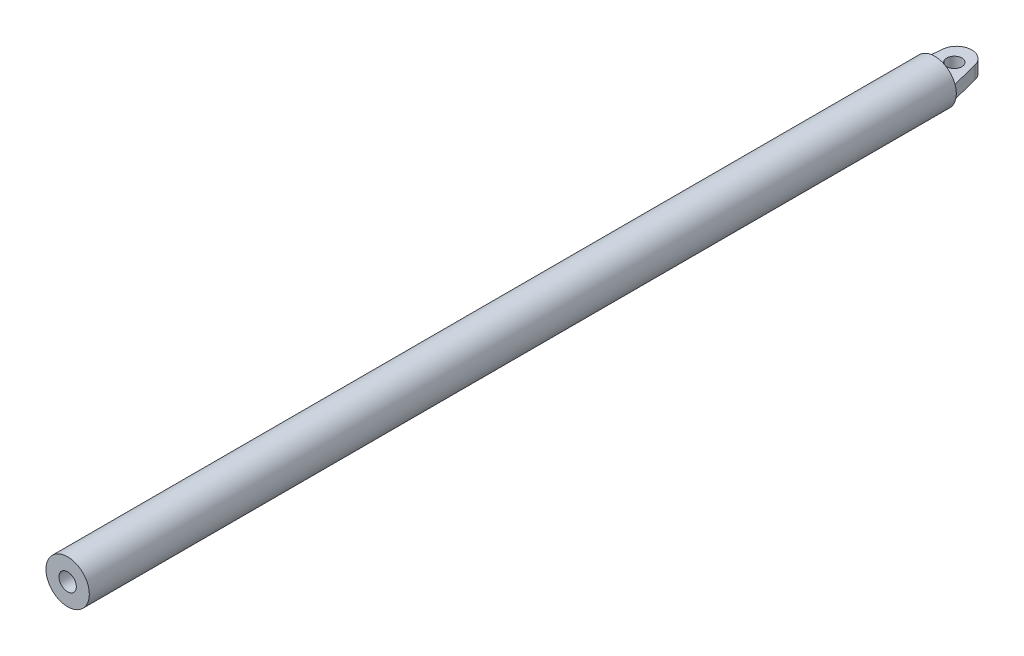
ISO-10303-21;
HEADER;
FILE_DESCRIPTION(('STEP AP214'),'2;1');
FILE_NAME('part.step','',(''),(''),'','','');
FILE_SCHEMA(('AUTOMOTIVE_DESIGN { 1 0 10303 214 1 1 1 1 }'));
ENDSEC;
DATA;
#1=APPLICATION_CONTEXT('core data for automotive mechanical design processes');
#2=APPLICATION_PROTOCOL_DEFINITION('international standard','automotive_design',2000,#1);
#3=PRODUCT_CONTEXT('',#1,'mechanical');
#4=PRODUCT('Part','Part','',(#3));
#5=PRODUCT_RELATED_PRODUCT_CATEGORY('part','',(#4));
#6=PRODUCT_DEFINITION_FORMATION('','',#4);
#7=PRODUCT_DEFINITION_CONTEXT('part definition',#1,'design');
#8=PRODUCT_DEFINITION('design','',#6,#7);
#9=PRODUCT_DEFINITION_SHAPE('','',#8);
#10=(LENGTH_UNIT() NAMED_UNIT(*) SI_UNIT(.MILLI.,.METRE.));
#11=(NAMED_UNIT(*) PLANE_ANGLE_UNIT() SI_UNIT($,.RADIAN.));
#12=(NAMED_UNIT(*) SI_UNIT($,.STERADIAN.) SOLID_ANGLE_UNIT());
#13=UNCERTAINTY_MEASURE_WITH_UNIT(LENGTH_MEASURE(1.E-05),#10,'distance_accuracy_value','');
#14=(GEOMETRIC_REPRESENTATION_CONTEXT(3) GLOBAL_UNCERTAINTY_ASSIGNED_CONTEXT((#13)) GLOBAL_UNIT_ASSIGNED_CONTEXT((#10,
#11,#12)) REPRESENTATION_CONTEXT('',''));
#15=CARTESIAN_POINT('',(0.,0.,0.));
#16=DIRECTION('',(0.,0.,1.));
#17=DIRECTION('',(1.,0.,0.));
#18=AXIS2_PLACEMENT_3D('',#15,#16,#17);
#19=CARTESIAN_POINT('',(-4.83861305777841,15.,-55.3975445891575));
#20=DIRECTION('',(0.,-1.,0.));
#21=DIRECTION('',(0.,0.,-1.));
#22=AXIS2_PLACEMENT_3D('',#19,#20,#21);
#23=PLANE('',#22);
#24=DIRECTION('',(0.999993507823482,0.,-0.00360337493019733));
#25=VECTOR('',#24,1.);
#26=CARTESIAN_POINT('',(-45.,15.,0.));
#27=LINE('',#26,#25);
#28=CARTESIAN_POINT('',(-45.,15.,0.));
#29=VERTEX_POINT('',#28);
#30=CARTESIAN_POINT('',(44.9988314120201,15.,-0.32430163828061));
#31=VERTEX_POINT('',#30);
#32=EDGE_CURVE('E103',#29,#31,#27,.T.);
#33=ORIENTED_EDGE('',*,*,#32,.T.);
#34=DIRECTION('',(-0.242420113613049,0.,-0.970171370694805));
#35=VECTOR('',#34,1.);
#36=CARTESIAN_POINT('',(29.1173849165398,15.,-63.8822485656143));
#37=LINE('',#36,#35);
#38=CARTESIAN_POINT('',(29.1173849165398,15.,-63.8822485656143));
#39=VERTEX_POINT('',#38);
#40=EDGE_CURVE('E98',#31,#39,#37,.T.);
#41=ORIENTED_EDGE('',*,*,#40,.T.);
#42=CARTESIAN_POINT('',(-4.83861305777841,15.,-55.3975445891575));
#43=DIRECTION('',(0.,1.,0.));
#44=DIRECTION('',(0.,0.,-1.));
#45=AXIS2_PLACEMENT_3D('',#42,#43,#44);
#46=CIRCLE('',#45,35.);
#47=CARTESIAN_POINT('',(-39.6958976744745,15.,-58.5550292131334));
#48=VERTEX_POINT('',#47);
#49=EDGE_CURVE('E101',#39,#48,#46,.T.);
#50=ORIENTED_EDGE('',*,*,#49,.T.);
#51=DIRECTION('',(-0.0902138463993087,0.,0.995922417619888));
#52=VECTOR('',#51,1.);
#53=CARTESIAN_POINT('',(-45.,15.,0.));
#54=LINE('',#53,#52);
#55=EDGE_CURVE('E69',#48,#29,#54,.T.);
#56=ORIENTED_EDGE('',*,*,#55,.T.);
#57=EDGE_LOOP('',(#33,#41,#50,#56));
#58=FACE_BOUND('',#57,.T.);
#59=CARTESIAN_POINT('',(0.,15.,-45.3243016382803));
#60=DIRECTION('',(0.,1.,0.));
#61=DIRECTION('',(0.,0.,1.));
#62=AXIS2_PLACEMENT_3D('',#59,#60,#61);
#63=CIRCLE('',#62,17.5);
#64=CARTESIAN_POINT('',(0.,15.,-27.8243016382803));
#65=VERTEX_POINT('',#64);
#66=EDGE_CURVE('E117',#65,#65,#63,.T.);
#67=ORIENTED_EDGE('',*,*,#66,.F.);
#68=EDGE_LOOP('',(#67));
#69=FACE_BOUND('',#68,.T.);
#70=ADVANCED_FACE('F51',(#58,#69),#23,.F.);
#71=CARTESIAN_POINT('',(-4.83861305777841,-15.,-55.3975445891575));
#72=DIRECTION('',(0.,-1.,0.));
#73=DIRECTION('',(0.,0.,-1.));
#74=AXIS2_PLACEMENT_3D('',#71,#72,#73);
#75=PLANE('',#74);
#76=DIRECTION('',(0.999993507823482,0.,-0.00360337493019733));
#77=VECTOR('',#76,1.);
#78=CARTESIAN_POINT('',(-45.,-15.,0.));
#79=LINE('',#78,#77);
#80=CARTESIAN_POINT('',(-45.,-15.,0.));
#81=VERTEX_POINT('',#80);
#82=CARTESIAN_POINT('',(44.9988314120201,-15.,-0.32430163828061));
#83=VERTEX_POINT('',#82);
#84=EDGE_CURVE('E113',#81,#83,#79,.T.);
#85=ORIENTED_EDGE('',*,*,#84,.F.);
#86=DIRECTION('',(-0.0902138463993087,0.,0.995922417619888));
#87=VECTOR('',#86,1.);
#88=CARTESIAN_POINT('',(-45.,-15.,0.));
#89=LINE('',#88,#87);
#90=CARTESIAN_POINT('',(-39.6958976744745,-15.,-58.5550292131334));
#91=VERTEX_POINT('',#90);
#92=EDGE_CURVE('E93',#91,#81,#89,.T.);
#93=ORIENTED_EDGE('',*,*,#92,.F.);
#94=CARTESIAN_POINT('',(-4.83861305777841,-15.,-55.3975445891575));
#95=DIRECTION('',(0.,1.,0.));
#96=DIRECTION('',(0.,0.,-1.));
#97=AXIS2_PLACEMENT_3D('',#94,#95,#96);
#98=CIRCLE('',#97,35.);
#99=CARTESIAN_POINT('',(29.1173849165398,-15.,-63.8822485656143));
#100=VERTEX_POINT('',#99);
#101=EDGE_CURVE('E85',#100,#91,#98,.T.);
#102=ORIENTED_EDGE('',*,*,#101,.F.);
#103=DIRECTION('',(-0.242420113613049,0.,-0.970171370694805));
#104=VECTOR('',#103,1.);
#105=CARTESIAN_POINT('',(29.1173849165398,-15.,-63.8822485656143));
#106=LINE('',#105,#104);
#107=EDGE_CURVE('E110',#83,#100,#106,.T.);
#108=ORIENTED_EDGE('',*,*,#107,.F.);
#109=EDGE_LOOP('',(#85,#93,#102,#108));
#110=FACE_BOUND('',#109,.T.);
#111=CARTESIAN_POINT('',(0.,-15.,-45.3243016382803));
#112=DIRECTION('',(0.,1.,0.));
#113=DIRECTION('',(0.,0.,1.));
#114=AXIS2_PLACEMENT_3D('',#111,#112,#113);
#115=CIRCLE('',#114,17.5);
#116=CARTESIAN_POINT('',(0.,-15.,-27.8243016382803));
#117=VERTEX_POINT('',#116);
#118=EDGE_CURVE('E128',#117,#117,#115,.T.);
#119=ORIENTED_EDGE('',*,*,#118,.T.);
#120=EDGE_LOOP('',(#119));
#121=FACE_BOUND('',#120,.T.);
#122=ADVANCED_FACE('F127',(#110,#121),#75,.T.);
#123=CARTESIAN_POINT('',(-45.,15.,0.));
#124=DIRECTION('',(-0.00360337493019733,0.,-0.999993507823482));
#125=DIRECTION('',(-0.999993507823482,0.,0.00360337493019733));
#126=AXIS2_PLACEMENT_3D('',#123,#124,#125);
#127=PLANE('',#126);
#128=ORIENTED_EDGE('',*,*,#84,.T.);
#129=DIRECTION('',(0.,-1.,0.));
#130=VECTOR('',#129,1.);
#131=CARTESIAN_POINT('',(44.9988314120201,15.,-0.32430163828061));
#132=LINE('',#131,#130);
#133=EDGE_CURVE('E12',#31,#83,#132,.T.);
#134=ORIENTED_EDGE('',*,*,#133,.F.);
#135=ORIENTED_EDGE('',*,*,#32,.F.);
#136=DIRECTION('',(0.,-1.,0.));
#137=VECTOR('',#136,1.);
#138=CARTESIAN_POINT('',(-45.,15.,0.));
#139=LINE('',#138,#137);
#140=EDGE_CURVE('E112',#29,#81,#139,.T.);
#141=ORIENTED_EDGE('',*,*,#140,.T.);
#142=EDGE_LOOP('',(#128,#134,#135,#141));
#143=FACE_BOUND('',#142,.T.);
#144=ADVANCED_FACE('F52',(#143),#127,.F.);
#145=CARTESIAN_POINT('',(29.1173849165398,15.,-63.8822485656143));
#146=DIRECTION('',(-0.970171370694805,0.,0.242420113613049));
#147=DIRECTION('',(0.242420113613049,0.,0.970171370694805));
#148=AXIS2_PLACEMENT_3D('',#145,#146,#147);
#149=PLANE('',#148);
#150=ORIENTED_EDGE('',*,*,#107,.T.);
#151=DIRECTION('',(0.,-1.,0.));
#152=VECTOR('',#151,1.);
#153=CARTESIAN_POINT('',(29.1173849165398,15.,-63.8822485656143));
#154=LINE('',#153,#152);
#155=EDGE_CURVE('E58',#39,#100,#154,.T.);
#156=ORIENTED_EDGE('',*,*,#155,.F.);
#157=ORIENTED_EDGE('',*,*,#40,.F.);
#158=ORIENTED_EDGE('',*,*,#133,.T.);
#159=EDGE_LOOP('',(#150,#156,#157,#158));
#160=FACE_BOUND('',#159,.T.);
#161=ADVANCED_FACE('F106',(#160),#149,.F.);
#162=CARTESIAN_POINT('',(-4.83861305777841,15.,-55.3975445891575));
#163=DIRECTION('',(0.,-1.,0.));
#164=DIRECTION('',(0.,0.,-1.));
#165=AXIS2_PLACEMENT_3D('',#162,#163,#164);
#166=CYLINDRICAL_SURFACE('',#165,35.);
#167=ORIENTED_EDGE('',*,*,#101,.T.);
#168=DIRECTION('',(0.,-1.,0.));
#169=VECTOR('',#168,1.);
#170=CARTESIAN_POINT('',(-39.6958976744745,15.,-58.5550292131334));
#171=LINE('',#170,#169);
#172=EDGE_CURVE('E107',#48,#91,#171,.T.);
#173=ORIENTED_EDGE('',*,*,#172,.F.);
#174=ORIENTED_EDGE('',*,*,#49,.F.);
#175=ORIENTED_EDGE('',*,*,#155,.T.);
#176=EDGE_LOOP('',(#167,#173,#174,#175));
#177=FACE_BOUND('',#176,.T.);
#178=ADVANCED_FACE('F108',(#177),#166,.T.);
#179=CARTESIAN_POINT('',(-45.,15.,0.));
#180=DIRECTION('',(0.995922417619888,0.,0.0902138463993087));
#181=DIRECTION('',(0.0902138463993087,0.,-0.995922417619888));
#182=AXIS2_PLACEMENT_3D('',#179,#180,#181);
#183=PLANE('',#182);
#184=ORIENTED_EDGE('',*,*,#92,.T.);
#185=ORIENTED_EDGE('',*,*,#140,.F.);
#186=ORIENTED_EDGE('',*,*,#55,.F.);
#187=ORIENTED_EDGE('',*,*,#172,.T.);
#188=EDGE_LOOP('',(#184,#185,#186,#187));
#189=FACE_BOUND('',#188,.T.);
#190=ADVANCED_FACE('F124',(#189),#183,.F.);
#191=CARTESIAN_POINT('',(0.,15.,-45.3243016382803));
#192=DIRECTION('',(0.,-1.,0.));
#193=DIRECTION('',(0.,0.,-1.));
#194=AXIS2_PLACEMENT_3D('',#191,#192,#193);
#195=CYLINDRICAL_SURFACE('',#194,17.5);
#196=ORIENTED_EDGE('',*,*,#66,.T.);
#197=EDGE_LOOP('',(#196));
#198=FACE_BOUND('',#197,.T.);
#199=ORIENTED_EDGE('',*,*,#118,.F.);
#200=EDGE_LOOP('',(#199));
#201=FACE_BOUND('',#200,.T.);
#202=ADVANCED_FACE('F136',(#198,#201),#195,.F.);
#203=CLOSED_SHELL('',(#70,#122,#144,#161,#178,#190,#202));
#204=MANIFOLD_SOLID_BREP('B2',#203);
#205=CARTESIAN_POINT('',(0.,0.,2000.));
#206=DIRECTION('',(0.,0.,-1.));
#207=DIRECTION('',(-1.,0.,0.));
#208=AXIS2_PLACEMENT_3D('',#205,#206,#207);
#209=CYLINDRICAL_SURFACE('',#208,50.);
#210=CARTESIAN_POINT('',(0.,0.,2000.));
#211=DIRECTION('',(0.,0.,1.));
#212=DIRECTION('',(1.,0.,0.));
#213=AXIS2_PLACEMENT_3D('',#210,#211,#212);
#214=CIRCLE('',#213,50.);
#215=CARTESIAN_POINT('',(50.,0.,2000.));
#216=VERTEX_POINT('',#215);
#217=EDGE_CURVE('E49',#216,#216,#214,.T.);
#218=ORIENTED_EDGE('',*,*,#217,.F.);
#219=EDGE_LOOP('',(#218));
#220=FACE_BOUND('',#219,.T.);
#221=CARTESIAN_POINT('',(0.,0.,0.));
#222=DIRECTION('',(0.,0.,1.));
#223=DIRECTION('',(1.,0.,0.));
#224=AXIS2_PLACEMENT_3D('',#221,#222,#223);
#225=CIRCLE('',#224,50.);
#226=CARTESIAN_POINT('',(50.,0.,0.));
#227=VERTEX_POINT('',#226);
#228=EDGE_CURVE('E230',#227,#227,#225,.T.);
#229=ORIENTED_EDGE('',*,*,#228,.T.);
#230=EDGE_LOOP('',(#229));
#231=FACE_BOUND('',#230,.T.);
#232=ADVANCED_FACE('F221',(#220,#231),#209,.T.);
#233=CARTESIAN_POINT('',(0.,0.,2000.));
#234=DIRECTION('',(0.,0.,1.));
#235=DIRECTION('',(1.,0.,0.));
#236=AXIS2_PLACEMENT_3D('',#233,#234,#235);
#237=PLANE('',#236);
#238=CARTESIAN_POINT('',(0.,0.,2000.));
#239=DIRECTION('',(0.,0.,1.));
#240=DIRECTION('',(1.,0.,0.));
#241=AXIS2_PLACEMENT_3D('',#238,#239,#240);
#242=CIRCLE('',#241,20.);
#243=CARTESIAN_POINT('',(20.,0.,2000.));
#244=VERTEX_POINT('',#243);
#245=EDGE_CURVE('E233',#244,#244,#242,.T.);
#246=ORIENTED_EDGE('',*,*,#245,.F.);
#247=EDGE_LOOP('',(#246));
#248=FACE_BOUND('',#247,.T.);
#249=ORIENTED_EDGE('',*,*,#217,.T.);
#250=EDGE_LOOP('',(#249));
#251=FACE_BOUND('',#250,.T.);
#252=ADVANCED_FACE('F255',(#248,#251),#237,.T.);
#253=CARTESIAN_POINT('',(0.,0.,0.));
#254=DIRECTION('',(0.,0.,1.));
#255=DIRECTION('',(1.,0.,0.));
#256=AXIS2_PLACEMENT_3D('',#253,#254,#255);
#257=PLANE('',#256);
#258=ORIENTED_EDGE('',*,*,#228,.F.);
#259=EDGE_LOOP('',(#258));
#260=FACE_BOUND('',#259,.T.);
#261=ADVANCED_FACE('F246',(#260),#257,.F.);
#262=CARTESIAN_POINT('',(0.,0.,2000.));
#263=DIRECTION('',(0.,0.,-1.));
#264=DIRECTION('',(-1.,0.,0.));
#265=AXIS2_PLACEMENT_3D('',#262,#263,#264);
#266=CYLINDRICAL_SURFACE('',#265,20.);
#267=ORIENTED_EDGE('',*,*,#245,.T.);
#268=EDGE_LOOP('',(#267));
#269=FACE_BOUND('',#268,.T.);
#270=CARTESIAN_POINT('',(0.,0.,30.));
#271=DIRECTION('',(0.,0.,1.));
#272=DIRECTION('',(1.,0.,0.));
#273=AXIS2_PLACEMENT_3D('',#270,#271,#272);
#274=CIRCLE('',#273,20.);
#275=CARTESIAN_POINT('',(20.,0.,30.));
#276=VERTEX_POINT('',#275);
#277=EDGE_CURVE('E236',#276,#276,#274,.T.);
#278=ORIENTED_EDGE('',*,*,#277,.F.);
#279=EDGE_LOOP('',(#278));
#280=FACE_BOUND('',#279,.T.);
#281=ADVANCED_FACE('F243',(#269,#280),#266,.F.);
#282=CARTESIAN_POINT('',(0.,0.,30.));
#283=DIRECTION('',(0.,0.,1.));
#284=DIRECTION('',(1.,0.,0.));
#285=AXIS2_PLACEMENT_3D('',#282,#283,#284);
#286=PLANE('',#285);
#287=ORIENTED_EDGE('',*,*,#277,.T.);
#288=EDGE_LOOP('',(#287));
#289=FACE_BOUND('',#288,.T.);
#290=ADVANCED_FACE('F245',(#289),#286,.T.);
#291=CLOSED_SHELL('',(#232,#252,#261,#281,#290));
#292=MANIFOLD_SOLID_BREP('B6',#291);
#293=ADVANCED_BREP_SHAPE_REPRESENTATION('',(#18,#204,#292),#14);
#294=SHAPE_DEFINITION_REPRESENTATION(#9,#293);
ENDSEC;
END-ISO-10303-21;
